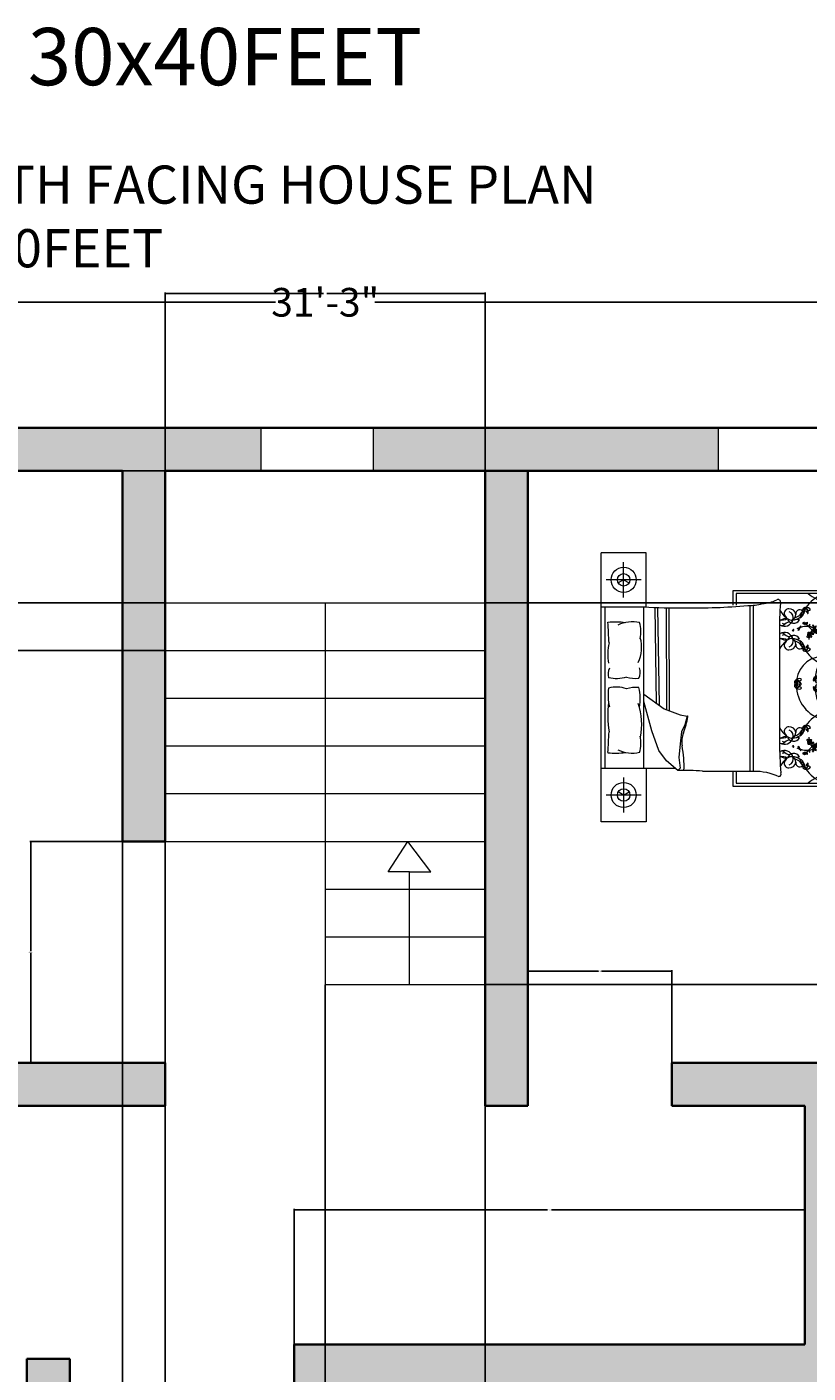
# Model space of a CAD drawing. Units: inches. Extents: x 8 to 486, y -516 to 97.
# Tile 4 of 5: x 162 to 326, y -185 to 97. Entities that reach past the tile are written whole.
import ezdxf

# ---------------------------------------------------------------- set-up
doc = ezdxf.new("R2010")
doc.units = ezdxf.units.IN
doc.header["$MEASUREMENT"] = 0
for name, color, linetype, lineweight in [('A-ANNO-DIMS', 2, 'Continuous', 18), ('A-ANNO-TEXT', 7, 'Continuous', 25), ('A-FLOR-STRS', 7, 'Continuous', 18), ('A-FURN', 8, 'Continuous', 18), ('A-GLAZ', 4, 'Continuous', 18), ('A-WALL', 7, 'Continuous', 35), ('A-WALL-PATT', 150, 'Continuous', 13)]:
    doc.layers.add(name, color=color, linetype=linetype, lineweight=lineweight)
doc.styles.get("Standard").update_dxf_attribs({"font": 'arial.ttf'})
doc.dimstyles.get("Standard").update_dxf_attribs({"dimtxt": 0.18, "dimasz": 0.18, "dimexe": 0.18, "dimexo": 0.0625, "dimgap": 0.09, "dimtad": 0, "dimtih": 1, "dimtoh": 1, "dimdec": 0, "dimzin": 0, "dimdsep": 46, "dimlunit": 3, "dimtxsty": 'Standard', "dimcen": 0.09, "dimadec": 0, "dimazin": 0, "dimtfac": 1, "dimtdec": 0, "dimtofl": 0, "dimtmove": 0, "dimatfit": 3, "dimfxl": 1, "dimtolj": 1, "dimtzin": 0, "dimarcsym": 0})

# ---------------------------------------------------------------- blocks, each defined once
blk = doc.blocks.new('*D1')
at = {"layer": 'A-ANNO-DIMS', "color": 0, "lineweight": -2, "transparency": 16777216}
for p, q in [((37.13, 12.8), (37.13, 39.25)), ((37.31, 39.07), (214.23, 39.07)), ((411.95, 39.07), (235.02, 39.07)), ((412.13, 12.8), (412.13, 39.25))]:
    blk.add_line(p, q, dxfattribs=at)
at = {"layer": 'A-ANNO-DIMS', "color": 0, "transparency": 16777216}
for points in [[(37.31, 39.1), (37.31, 39.04), (37.13, 39.07)], [(411.95, 39.1), (411.95, 39.04), (412.13, 39.07)]]:
    blk.add_solid(points, dxfattribs=at)
at = {"layer": 'Defpoints', "color": 0, "transparency": 16777216}
for p in [(412.13, 39.07), (37.13, 12.74), (412.13, 12.74)]:
    blk.add_point(p, dxfattribs=at)
at = {"layer": 'A-ANNO-DIMS', "color": 0, "transparency": 16777216, "insert": (224.63, 39.07), "char_height": 6, "attachment_point": 5}
blk.add_mtext('\\A1;31\'-3"', dxfattribs=at)
blk = doc.blocks.new('BED-DOUBLE')
for p, q in [((0, 0), (0, 56.34)), ((4.7, 47.03), (4.7, 54.39)), ((8.38, 50.71), (1.01, 50.71)), ((27.62, 45.39), (27.62, 48.51)), ((27.62, 48.51), (47.92, 48.51)), ((47.92, 48.51), (47.92, 7.44)), ((28.27, 47.86), (28.27, 45.37)), ((47.26, 47.86), (28.27, 47.86)), ((31.13, 45.33), (31.13, 10.62)), ((31.84, 45.38), (31.84, 10.62)), ((47.26, 8.09), (47.26, 47.86)), ((0.72, 45.07), (0.72, 11.27)), ((8.9, 11.27), (8.9, 45.07)), ((11.24, 44.92), (11.53, 24.86)), ((11.82, 44.9), (12.11, 24.44)), ((13.6, 44.87), (13.68, 23.48)), ((14.18, 44.87), (14.26, 23.26)), ((41.55, 42.31), (40.91, 42.43)), ((37.37, 39.61), (37.37, 16.73)), ((41.55, 38.37), (40.91, 38.24)), ((8.9, 26.75), (13.2, 23.66)), ((10.58, 19.09), (8.9, 25.24)), ((13.2, 23.66), (16.51, 22.4)), ((16.51, 22.4), (17.99, 22.17)), ((17.54, 20.35), (16.85, 18.87)), ((17.99, 22.17), (17.54, 20.35)), ((12.06, 14.99), (10.58, 19.09)), ((16.85, 18.87), (16.51, 16.36)), ((41.55, 17.58), (40.91, 17.7)), ((13.66, 12.82), (12.06, 14.99)), ((16.51, 16.36), (16.28, 13.5)), ((16.05, 10.76), (13.66, 12.82)), ((16.28, 13.5), (16.51, 11.22)), ((41.55, 13.64), (40.91, 13.52)), ((0, 11.27), (15.46, 11.27)), ((4.7, 9.31), (4.7, 1.95)), ((16.51, 11.22), (16.05, 10.76)), ((27.62, 7.44), (27.62, 10.62)), ((28.27, 10.62), (28.27, 8.09)), ((47.92, 7.44), (27.62, 7.44)), ((28.27, 8.09), (47.26, 8.09)), ((8.38, 5.63), (1.01, 5.63))]:
    blk.add_line(p, q)
for points in [[(0, 45.07), (9.39, 45.07), (9.39, 56.34), (0, 56.34)], [(4.7, 50.71), (3.56, 50.05)], [(4.7, 50.71), (5.83, 50.05)], [(9.39, 11.27), (9.39, 0), (0, 0)], [(4.7, 5.63), (3.56, 6.29)], [(4.7, 5.63), (5.83, 6.29)]]:
    blk.add_lwpolyline(points)
for points in [[(30.69, 45.31, 0.056112), (33.79, 45.72, 0.095341), (36.78, 46.51)], [(1.4, 41.84, -0.074897), (5.08, 41.77, 0.472817)], [(5.29, 30.31, -0.14099), (1.54, 30.2, -0.235245)], [(5.29, 27.91, 0.14099), (1.54, 28.02, 0.235245)], [(1.4, 14.5, 0.074897), (5.08, 14.57, -0.472817)], [(21.21, 10.65, 0.001242), (31.9, 10.62, -0.127202), (37.23, 9.49)]]:
    blk.add_lwpolyline(points, format="xyb")
for centre, radius in [((4.7, 50.71), 2.63), ((4.7, 50.71), 1.31), ((45.1, 39.99), 0.143), ((43.59, 39.05), 0.143), ((43.59, 16.9), 0.143), ((45.1, 15.96), 0.143), ((4.7, 5.63), 2.63), ((4.7, 5.63), 1.31)]:
    blk.add_circle(centre, radius)
for centre, radius, start, end in [((19.47, 176.89), 132.06, 269.1145, 274.8735), ((37.06, 46.09), 0.514, 336.5219, 123.8264), ((92.17, 41.33), 54.82, 175.2402, 181.8035), ((48.98, 40.75), 7.36, 111.4092, 145.6135), ((48.25, 53.34), 7.36, 228.1144, 262.255), ((49.24, 49.64), 3.59, 209.8884, 236.5383), ((48.41, 47.64), 2.99, 221.0454, 247.4453), ((46.8, 55.83), 10.18, 266.3481, 272.5919), ((49.91, 50.93), 4.47, 223.5186, 233.6964), ((15.79, 146.07), 101.24, 266.1, 270.9282), ((37.79, 44.6), 2.33, 259.249, 301.1782), ((41.34, 46.16), 4.26, 203.6453, 236.3329), ((38.8, 40.44), 2.17, 85.2696, 124.215), ((39.29, 43.68), 0.951, 88.9462, 185.5144), ((39.99, 43.97), 1.69, 193.079, 274.7067), ((40.34, 43), 1.4, 196.8663, 330.0915), ((39.43, 43.29), 1.35, 7.1143, 95.0551), ((38.92, 42.76), 1.31, 338.5779, 68.4181), ((39.13, 43.52), 1.64, 305.9599, 357.6409), ((39.95, 45.3), 3.02, 273.4924, 303.7117), ((39.73, 45.27), 2.66, 288.2955, 328.7386), ((41.6, 43.6), 0.846, 19.1312, 189.736), ((41.34, 43.8), 1.06, 285.6955, 4.031), ((42.75, 42.66), 1.12, 128.4175, 173.8338), ((42.51, 43.77), 0.518, 126.7319, 206.0245), ((42.76, 44.31), 0.61, 76.272, 177.0484), ((41.84, 45.56), 1.26, 284.7031, 328.6173), ((43.59, 43.96), 1.16, 125.7657, 194.5347), ((37.88, 46.02), 5.15, 332.8176, 347.4827), ((43.08, 44.11), 0.816, 20.9613, 102.2885), ((43.52, 44.92), 0.614, 181.7131, 301.5367), ((41.51, 43.68), 1.86, 2.0648, 41.1598), ((42.63, 44.37), 0.602, 316.2238, 62.3173), ((42.98, 44.02), 0.048, 20.2667, 316.2271), ((43.23, 43.75), 0.0444, 52.0591, 168.5166), ((43.28, 43.74), 0.0914, 168.5166, 2.0648), ((-534.78, 10.78), 537.08, 2.8502, 3.3148), ((6.56, 34.66), 7.26, 78.2417, 114.8684), ((0.75, 39.83), 7.55, 348.9631, 14.8961), ((37.99, 41.7), 0.679, 196.6343, 225.5483), ((37.99, 41.7), 0.679, 127.675, 162.5814), ((38.39, 42.79), 1.8, 240.8249, 340.7178), ((37.86, 41.99), 0.843, 246.1646, 318.4347), ((38.39, 37.89), 1.8, 19.2822, 119.1751), ((37.86, 38.68), 0.843, 41.5653, 113.8354), ((38.72, 43.06), 1.62, 240.0851, 262.564), ((39.35, 40.67), 1.16, 74.8529, 138.4347), ((39.75, 42.12), 0.35, 254.8529, 12.6959), ((38.8, 40.44), 2.17, 53.6555, 57.2989), ((40.21, 40.19), 0.177, 169.5864, 349.5616), ((40.28, 40.18), 0.109, 349.5616, 167.2949), ((43.11, 36.27), 4.67, 110.1059, 116.9968), ((41.55, 40.12), 0.296, 129.5056, 182.6421), ((40.7, 40.8), 0.89, 308.4388, 328.836), ((40.54, 41.53), 1.59, 296.5064, 305.3102), ((40.53, 40.71), 0.905, 336.3901, 344.4871), ((41.52, 40.48), 0.115, 83.9457, 185.6216), ((41.06, 40.58), 0.472, 328.836, 0.8141), ((41.3, 40.45), 0.27, 306.5232, 32.4668), ((41.62, 40.66), 0.115, 112.5583, 214.2343), ((41.55, 40.86), 0.27, 265.7131, 351.6568), ((41.31, 41.01), 0.472, 297.3659, 329.344), ((40.95, 41.42), 0.905, 313.6929, 321.7899), ((41.96, 40.8), 0.296, 115.5379, 168.6744), ((40.95, 41.22), 0.89, 329.344, 349.7412), ((43.11, 36.27), 4.67, 86.1723, 106.4158), ((40.24, 41.02), 1.59, 352.8698, 1.6736), ((42.35, 41.59), 0.111, 125.0752, 284.7644), ((42.52, 41.63), 0.239, 127.3642, 168.4363), ((42.33, 41.83), 0.345, 277.4968, 341.2737), ((42.6, 41.67), 0.137, 88.1325, 178.8919), ((42.88, 41.52), 0.297, 136.3462, 189.6513), ((42.71, 41.49), 0.124, 189.6513, 312.3208), ((42.74, 41.83), 0.143, 183.2768, 356.7232), ((43.19, 41.58), 0.47, 164.2829, 186.9148), ((42.63, 41.57), 0.235, 312.3208, 40.2111), ((43.13, 41.84), 0.333, 201.6382, 274.947), ((42.69, 41.38), 0.436, 42.3896, 66.5724), ((47.08, 44.83), 5.35, 217.9541, 226.8459), ((43, 41.64), 0.237, 10.9597, 52.2379), ((43.15, 41.62), 0.11, 274.947, 37.5263), ((43.38, 40.15), 0.654, 253.6301, 325.4631), ((43.56, 39.24), 0.463, 82.0748, 142.6895), ((43.51, 39.88), 0.475, 228.342, 274.9894), ((43.52, 40.99), 0.115, 112.5583, 214.2343), ((43.45, 41.2), 0.27, 265.7131, 351.6568), ((43.21, 41.35), 0.472, 297.3659, 329.344), ((43.23, 38.6), 2.34, 60.7959, 85.244), ((38.25, 35.23), 7.7, 37.8256, 47.7588), ((42.85, 41.75), 0.905, 313.6929, 321.7899), ((43.52, 39.8), 0.398, 273.8774, 357.1501), ((43.85, 41.13), 0.296, 115.5379, 168.6744), ((42.85, 41.56), 0.89, 329.344, 349.7412), ((43.68, 40.08), 0.385, 262.0748, 308.2393), ((42.14, 41.35), 1.59, 352.8698, 1.6736), ((46.34, 38.35), 2.81, 156.1523, 156.9499), ((43.86, 39.35), 0.142, 44.3732, 121.9501), ((44.3, 39.69), 0.398, 181.4625, 249.4747), ((46.34, 38.35), 2.81, 130.182, 149.456), ((44.23, 40), 0.385, 215.1128, 261.2773), ((44.54, 39.98), 0.654, 197.889, 269.722), ((44.1, 39.16), 0.463, 20.6625, 81.2773), ((44.37, 41.03), 0.16, 33.0979, 123.1364), ((40.84, 38.77), 4.19, 31.1156, 34.8118), ((44.14, 40.76), 0.434, 2.3172, 70.5201), ((44.79, 39.95), 0.463, 139.3812, 199.9959), ((43.93, 40.29), 0.654, 310.9365, 22.7695), ((44.23, 40.25), 0.475, 285.6484, 332.2957), ((44.5, 40.65), 0.125, 135.7354, 318.1297), ((44.29, 40.86), 0.166, 315.7354, 31.1156), ((44.15, 40.5), 0.385, 319.3812, 5.5456), ((44.59, 40.65), 0.125, 68.2452, 250.6395), ((44.3, 40.81), 0.374, 352.6008, 57.1845), ((45.64, 38.3), 2.5, 111.7087, 116.2181), ((43.23, 38.6), 2.34, 47.5083, 55.9967), ((44.66, 40.89), 0.374, 252.8042, 349.6943), ((44.3, 40.22), 0.398, 331.1838, 51.6792), ((44.71, 39.75), 0.111, 125.0752, 284.7644), ((44.7, 40.92), 0.166, 248.2452, 323.6254), ((44.88, 39.79), 0.239, 93.635, 168.4363), ((44.55, 41.02), 0.434, 291.7087, 3.0299), ((44.85, 40.17), 0.141, 138.2946, 276.2474), ((44.69, 39.98), 0.345, 277.4968, 341.2737), ((44.9, 40.15), 0.196, 358.5719, 143.8954), ((41.46, 43.31), 4.19, 323.6254, 327.3216), ((44.97, 39.82), 0.137, 88.1325, 178.8919), ((45.02, 40.3), 0.197, 208.8493, 269.9355), ((44.85, 40.26), 0.226, 274.2123, 318.1587), ((45.24, 39.68), 0.297, 136.3462, 189.6513), ((45.07, 39.65), 0.124, 189.6513, 312.3208), ((44.89, 40.92), 0.16, 325.6077, 55.6462), ((45.55, 39.73), 0.47, 164.2829, 186.9148), ((45.54, 40.03), 0.452, 121.9501, 165.2442), ((45, 39.73), 0.235, 312.3208, 40.2111), ((45.5, 39.99), 0.333, 201.6382, 274.947), ((45.23, 40.2), 0.095, 262.868, 7.094), ((45.05, 39.54), 0.436, 42.3896, 66.5724), ((45.21, 40.28), 0.283, 278.5614, 22.5914), ((45.37, 39.79), 0.237, 10.9597, 118.7804), ((45.37, 40.29), 0.142, 44.3732, 121.9501), ((45.52, 39.77), 0.11, 274.947, 37.5263), ((11.26, 35.15), 9.9, 166.3427, 191.1841), ((1.3, 36.57), 7.17, 333.8761, 16.1746), ((37.99, 38.97), 0.679, 134.4517, 156.7144), ((37.99, 38.97), 0.679, 203.2856, 232.325), ((37.79, 36.08), 2.33, 58.8218, 100.2867), ((41.34, 34.52), 4.26, 123.6671, 158.5059), ((38.8, 40.23), 2.17, 235.785, 274.7304), ((38.72, 37.62), 1.62, 97.436, 119.9149), ((39.99, 36.71), 1.69, 85.2933, 166.921), ((39.29, 37), 0.951, 174.4856, 271.0538), ((39.35, 40.01), 1.16, 221.5653, 285.1471), ((40.34, 37.67), 1.4, 29.9085, 163.1337), ((39.43, 37.39), 1.35, 264.9449, 352.8857), ((38.92, 37.92), 1.31, 291.5819, 21.4221), ((39.75, 38.56), 0.35, 347.3041, 105.1471), ((38.8, 40.23), 2.17, 302.7011, 306.3445), ((39.13, 37.16), 1.64, 2.3591, 54.0401), ((39.95, 35.38), 3.02, 56.2883, 86.5076), ((39.73, 35.4), 2.66, 31.2614, 71.7045), ((41.6, 37.08), 0.846, 170.264, 340.8688), ((42.75, 38.01), 1.12, 186.1662, 231.5825), ((41.34, 36.88), 1.06, 355.969, 74.3045), ((42.51, 36.91), 0.518, 153.9755, 233.2681), ((43.59, 36.72), 1.16, 165.4653, 234.2343), ((37.88, 34.66), 5.15, 12.5173, 27.1824), ((41.51, 37), 1.86, 318.8402, 357.9352), ((42.63, 36.3), 0.602, 297.6827, 43.7762), ((43.01, 36.67), 0.0796, 43.7762, 339.7183), ((43.2, 38.81), 0.111, 125.0752, 284.7644), ((43.37, 38.85), 0.239, 93.635, 168.4363), ((43.28, 36.93), 0.0914, 357.9352, 191.4834), ((43.23, 36.92), 0.0444, 191.4834, 307.9409), ((43.34, 39.23), 0.141, 138.2946, 276.2474), ((43.39, 39.21), 0.196, 358.5719, 143.8954), ((43.18, 39.05), 0.345, 277.4968, 341.2737), ((43.46, 38.88), 0.137, 88.1325, 178.8919), ((43.51, 39.36), 0.197, 208.8493, 269.9355), ((43.34, 39.32), 0.226, 274.2123, 318.1587), ((43.73, 38.74), 0.297, 136.3462, 189.6513), ((43.56, 38.71), 0.124, 189.6513, 312.3208), ((46.34, 38.35), 2.81, 175.2415, 182.8929), ((44.04, 38.79), 0.47, 164.2829, 186.9148), ((44.03, 39.09), 0.452, 121.9501, 165.2442), ((43.49, 38.79), 0.235, 312.3208, 40.2111), ((43.98, 39.06), 0.333, 201.6382, 274.947), ((43.71, 39.26), 0.095, 262.868, 7.094), ((43.54, 38.6), 0.436, 42.3896, 66.5724), ((43.7, 39.34), 0.283, 278.5614, 22.5914), ((43.86, 38.86), 0.237, 10.9597, 118.7804), ((44, 38.83), 0.11, 274.947, 37.5263), ((44.34, 39.76), 0.475, 248.3627, 295.0101), ((46.55, 28.98), 5.69, 82.8636, 171.8197), ((42.76, 36.36), 0.61, 182.9516, 283.728), ((41.84, 35.12), 1.26, 31.3827, 75.2969), ((43.52, 35.75), 0.614, 58.4633, 178.2869), ((43.08, 36.57), 0.816, 257.7115, 339.0387), ((48.98, 39.93), 7.36, 214.3865, 248.5908), ((46.95, 32.74), 1.32, 76.3898, 169.0739), ((48.41, 33.04), 2.99, 112.5547, 138.9546), ((46.8, 24.84), 10.18, 87.4081, 93.6519), ((4.21, 30.97), 2.79, 153.3437, 196.1026), ((5.19, 31.35), 2.99, 335.0183, 18.5407), ((52.19, 29.78), 7.36, 152.5854, 175.5377), ((46.77, 31.74), 1.67, 72.8609, 131.9049), ((46.03, 29.72), 3.29, 68.117, 96.6195), ((51.13, 31.84), 4.05, 162.9798, 196.4569), ((7.17, 36.95), 6.9, 254.1707, 275.9871), ((41.09, 29.2), 0.61, 106.1963, 206.9726), ((41.09, 28.62), 0.61, 153.0274, 253.8037), ((39.66, 29.82), 1.26, 314.6273, 358.5415), ((39.66, 28), 1.26, 1.4585, 45.3727), ((41.98, 29.31), 1.16, 155.6899, 224.4589), ((41.98, 28.51), 1.16, 135.5411, 204.3101), ((41.47, 29.19), 0.816, 50.8855, 132.2127), ((41.44, 30.11), 0.614, 211.6373, 331.4609), ((40.94, 29.19), 0.602, 346.148, 92.2415), ((40.32, 28.03), 1.86, 31.989, 71.0841), ((36.01, 28.25), 5.15, 2.7418, 17.407), ((36.01, 29.58), 5.15, 342.593, 357.2582), ((40.32, 29.8), 1.86, 288.9159, 328.011), ((40.94, 28.64), 0.602, 267.7585, 13.852), ((41.44, 27.71), 0.614, 28.5391, 148.3627), ((41.42, 29.06), 0.048, 50.1909, 346.0209), ((41.45, 28.76), 0.0796, 13.852, 309.9245), ((41.82, 28.97), 0.0914, 198.4408, 31.989), ((41.77, 28.95), 0.0444, 81.9833, 198.4408), ((41.82, 28.86), 0.0914, 328.011, 161.5592), ((41.77, 28.87), 0.0444, 161.5592, 278.0167), ((45.03, 29.77), 0.61, 106.1963, 206.9726), ((45.03, 28.06), 0.61, 153.0274, 253.8037), ((43.6, 30.38), 1.26, 314.6273, 358.5415), ((43.6, 27.44), 1.26, 1.4585, 45.3727), ((45.92, 29.87), 1.16, 155.6899, 224.4589), ((45.92, 27.95), 1.16, 135.5411, 204.3101), ((45.41, 29.75), 0.816, 50.8855, 132.2127), ((45.38, 30.68), 0.614, 211.6373, 331.4609), ((44.26, 28.59), 1.86, 31.989, 71.0841), ((39.95, 28.81), 5.15, 2.7418, 17.407), ((44.88, 29.75), 0.602, 346.148, 92.2415), ((39.95, 29.01), 5.15, 342.593, 357.2582), ((44.26, 29.23), 1.86, 288.9159, 328.011), ((44.88, 28.07), 0.602, 267.7585, 13.852), ((45.36, 29.62), 0.048, 50.1909, 346.0209), ((45.39, 28.2), 0.0796, 13.852, 309.9245), ((45.76, 29.53), 0.0914, 198.4408, 31.989), ((45.71, 29.52), 0.0444, 81.9833, 198.4408), ((45.76, 28.3), 0.0914, 328.011, 161.5592), ((45.71, 28.31), 0.0444, 161.5592, 278.0167), ((53.22, 30.24), 5.98, 174.3643, 175.6213), ((57.31, 27.08), 10.69, 160.0972, 160.2783), ((11.47, 26.54), 10.04, 171.5249, 193.96), ((7.17, 21.26), 6.9, 84.0129, 105.8293), ((-1.76, 25.79), 9.94, 349.8617, 13.6238), ((41.47, 28.64), 0.816, 227.7873, 309.1145), ((48.25, 28.61), 7.36, 184.4623, 262.255), ((45.38, 27.15), 0.614, 28.5391, 148.3627), ((45.41, 28.08), 0.816, 227.7873, 309.1145), ((52.19, 28.04), 7.36, 184.4623, 207.4146), ((51.13, 25.99), 4.05, 163.5431, 197.0202), ((53.22, 27.59), 5.98, 184.3787, 185.6357), ((57.31, 30.74), 10.69, 199.7217, 199.9028), ((21.79, 22.22), 20.43, 172.2196, 189.497), ((-4.62, 20.49), 13.1, 348.0397, 19.2615), ((48.98, 16.02), 7.36, 111.4092, 145.6135), ((49.24, 24.92), 3.59, 181.272, 236.5383), ((51.16, 28.56), 6.65, 214.0123, 234.053), ((49.91, 26.21), 4.47, 197.8504, 233.6964), ((-3.3, 26.09), 21.85, 340.1194, 349.3383), ((18.04, 22.05), 0.136, 358.8623, 109.7536), ((41.34, 21.43), 4.26, 201.4941, 236.3329), ((39.29, 18.95), 0.951, 88.9462, 185.5144), ((39.43, 18.56), 1.35, 7.1143, 95.0551), ((42.76, 19.58), 0.61, 76.272, 177.0484), ((41.84, 20.83), 1.26, 284.7031, 328.6173), ((43.59, 19.23), 1.16, 125.7657, 194.5347), ((37.88, 21.29), 5.15, 332.8176, 347.4827), ((43.08, 19.38), 0.816, 20.9613, 102.2885), ((42.63, 19.64), 0.602, 316.2238, 62.3173), ((41.51, 18.95), 1.86, 2.0648, 41.1598), ((43.52, 20.19), 0.614, 181.7131, 301.5367), ((46.8, 31.1), 10.18, 266.3481, 272.5919), ((48.41, 22.91), 2.99, 221.0454, 247.4453), ((-534.78, 45.56), 537.08, 356.6852, 357.1498), ((0.75, 16.51), 7.55, 345.1039, 11.0369), ((21.45, 16.81), 4.59, 156.2616, 191.3392), ((37.79, 19.87), 2.33, 259.7133, 301.1782), ((37.99, 16.98), 0.679, 127.675, 156.7144), ((38.39, 18.06), 1.8, 240.8249, 340.7178), ((38.8, 15.72), 2.17, 85.2696, 124.215), ((38.72, 18.33), 1.62, 240.0851, 262.564), ((39.99, 19.24), 1.69, 193.079, 274.7067), ((39.35, 15.94), 1.16, 74.8529, 138.4347), ((40.34, 18.28), 1.4, 196.8663, 330.0915), ((38.92, 18.03), 1.31, 338.5779, 68.4181), ((39.75, 17.39), 0.35, 254.8529, 12.6959), ((38.8, 15.72), 2.17, 53.6555, 57.2989), ((39.13, 18.79), 1.64, 305.9599, 357.6409), ((39.95, 20.57), 3.02, 273.4924, 303.7117), ((39.73, 20.54), 2.66, 288.2955, 328.7386), ((41.6, 18.87), 0.846, 19.1312, 189.736), ((41.34, 19.07), 1.06, 285.6955, 4.031), ((42.75, 17.93), 1.12, 128.4175, 173.8338), ((42.51, 19.04), 0.518, 126.7319, 206.0245), ((42.98, 19.29), 0.048, 20.2667, 316.2271), ((43.2, 17.14), 0.111, 75.2356, 234.9248), ((43.37, 17.09), 0.239, 191.5637, 266.365), ((43.23, 19.02), 0.0444, 52.0591, 168.5166), ((43.28, 19.02), 0.0914, 168.5166, 2.0648), ((43.18, 16.9), 0.345, 18.7263, 82.5032), ((43.46, 17.06), 0.137, 181.1081, 271.8675), ((43.73, 17.21), 0.297, 170.3487, 223.6538), ((43.56, 17.24), 0.124, 47.6792, 170.3487), ((46.34, 17.59), 2.81, 177.1071, 184.7585), ((44.04, 17.15), 0.47, 173.0852, 195.7171), ((43.49, 17.16), 0.235, 319.7889, 47.6792), ((43.98, 16.89), 0.333, 85.053, 158.3618), ((43.54, 17.35), 0.436, 293.4276, 317.6104), ((43.86, 17.09), 0.237, 241.2196, 349.0403), ((44, 17.11), 0.11, 322.4737, 85.053), ((6.56, 21.68), 7.26, 245.1316, 281.7583), ((-3.9, 11.73), 21.26, 357.4519, 11.3392), ((96.02, 16.06), 58.65, 179.3433, 185.6887), ((37.99, 16.98), 0.679, 203.229, 225.5483), ((37.99, 14.24), 0.679, 134.4517, 153.558), ((37.86, 17.26), 0.843, 246.1646, 318.4347), ((38.39, 13.16), 1.8, 19.2822, 119.1751), ((37.86, 13.96), 0.843, 41.5653, 113.8354), ((38.72, 12.89), 1.62, 97.436, 119.9149), ((39.35, 15.28), 1.16, 221.5653, 285.1471), ((40.34, 12.94), 1.4, 29.9085, 163.1337), ((39.75, 13.83), 0.35, 347.3041, 105.1471), ((40.21, 15.76), 0.177, 10.4384, 190.4136), ((40.28, 15.77), 0.109, 192.7051, 10.4384), ((43.11, 19.68), 4.67, 243.0032, 249.8941), ((40.7, 15.15), 0.89, 31.164, 51.5612), ((41.55, 15.83), 0.296, 177.3579, 230.4944), ((40.54, 14.42), 1.59, 54.6898, 63.4936), ((40.53, 15.24), 0.905, 15.5129, 23.6099), ((41.52, 15.47), 0.115, 174.3784, 276.0543), ((41.3, 15.5), 0.27, 327.5332, 53.4768), ((41.06, 15.36), 0.472, 359.1859, 31.164), ((41.62, 15.29), 0.115, 145.7657, 247.4417), ((41.55, 15.09), 0.27, 8.3432, 94.2869), ((41.31, 14.94), 0.472, 30.656, 62.6341), ((40.95, 14.53), 0.905, 38.2101, 46.3071), ((41.96, 15.15), 0.296, 191.3256, 244.4621), ((40.95, 14.72), 0.89, 10.2588, 30.656), ((43.11, 19.68), 4.67, 253.5842, 273.8277), ((40.24, 14.93), 1.59, 358.3264, 7.1302), ((42.35, 14.36), 0.111, 75.2356, 234.9248), ((42.52, 14.31), 0.239, 191.5637, 232.6358), ((42.33, 14.12), 0.345, 18.7263, 82.5032), ((42.6, 14.28), 0.137, 181.1081, 271.8675), ((42.88, 14.43), 0.297, 170.3487, 223.6538), ((42.71, 14.46), 0.124, 47.6792, 170.3487), ((42.74, 14.11), 0.143, 3.2768, 176.7232), ((43.19, 14.37), 0.47, 173.0852, 195.7171), ((42.63, 14.37), 0.235, 319.7889, 47.6792), ((43.13, 14.11), 0.333, 85.053, 158.3618), ((42.69, 14.57), 0.436, 293.4276, 317.6104), ((47.08, 11.12), 5.35, 133.1541, 142.0459), ((43, 14.31), 0.237, 307.7621, 349.0403), ((43.15, 14.33), 0.11, 322.4737, 85.053), ((43.51, 16.07), 0.475, 85.0106, 131.658), ((43.38, 15.8), 0.654, 34.5369, 106.3699), ((43.56, 16.71), 0.463, 217.3105, 277.9252), ((43.34, 16.72), 0.141, 83.7526, 221.7054), ((43.39, 16.74), 0.196, 216.1046, 1.4281), ((43.51, 16.58), 0.197, 90.0645, 151.1507), ((43.34, 16.63), 0.226, 41.8413, 85.7877), ((43.52, 14.96), 0.115, 145.7657, 247.4417), ((38.25, 20.72), 7.7, 312.2412, 322.1744), ((43.23, 17.35), 2.34, 274.756, 299.2041), ((43.45, 14.75), 0.27, 8.3432, 94.2869), ((43.21, 14.6), 0.472, 30.656, 62.6341), ((42.85, 14.2), 0.905, 38.2101, 46.3071), ((43.52, 16.15), 0.398, 2.8499, 86.1226), ((43.85, 14.81), 0.296, 191.3256, 244.4621), ((44.03, 16.86), 0.452, 194.7558, 238.0499), ((42.85, 14.39), 0.89, 10.2588, 30.656), ((43.68, 15.87), 0.385, 51.7607, 97.9252), ((43.71, 16.68), 0.095, 352.906, 97.132), ((42.14, 14.59), 1.59, 358.3264, 7.1302), ((43.7, 16.6), 0.283, 337.4086, 81.4386), ((46.34, 17.59), 2.81, 203.0501, 203.8477), ((43.86, 16.59), 0.142, 238.0499, 315.6268), ((44.3, 16.26), 0.398, 110.5253, 178.5375), ((44.54, 15.97), 0.654, 90.278, 162.111), ((44.23, 15.95), 0.385, 98.7227, 144.8872), ((46.34, 17.59), 2.81, 210.544, 229.818), ((44.34, 16.19), 0.475, 64.9899, 111.6373), ((44.1, 16.78), 0.463, 278.7227, 339.3375), ((44.14, 15.19), 0.434, 289.4799, 357.6828), ((40.84, 17.17), 4.19, 325.1882, 328.8844), ((44.37, 14.91), 0.16, 236.8636, 326.9021), ((44.79, 15.99), 0.463, 160.0041, 220.6188), ((43.93, 15.66), 0.654, 337.2305, 49.0635), ((44.23, 15.7), 0.475, 27.7043, 74.3516), ((44.5, 15.3), 0.125, 41.8703, 224.2646), ((44.29, 15.09), 0.166, 328.8844, 44.2646), ((44.15, 15.44), 0.385, 354.4544, 40.6188), ((44.59, 15.29), 0.125, 109.3605, 291.7548), ((44.3, 15.14), 0.374, 302.8155, 7.3992), ((45.64, 17.65), 2.5, 243.7819, 248.2913), ((43.23, 17.35), 2.34, 304.0033, 312.4917), ((44.3, 15.72), 0.398, 308.3208, 28.8162), ((44.66, 15.06), 0.374, 10.3057, 107.1958), ((44.71, 16.2), 0.111, 75.2356, 234.9248), ((44.7, 15.02), 0.166, 36.3746, 111.7548), ((44.88, 16.16), 0.239, 191.5637, 266.365), ((44.85, 15.78), 0.141, 83.7526, 221.7054), ((44.55, 14.92), 0.434, 356.9701, 68.2913), ((44.69, 15.96), 0.345, 18.7263, 82.5032), ((44.9, 15.8), 0.196, 216.1046, 1.4281), ((44.97, 16.12), 0.137, 181.1081, 271.8675), ((41.46, 12.64), 4.19, 32.6784, 36.3746), ((45.02, 15.65), 0.197, 90.0645, 151.1507), ((44.85, 15.69), 0.226, 41.8413, 85.7877), ((45.07, 16.3), 0.124, 47.6792, 170.3487), ((45.24, 16.27), 0.297, 170.3487, 223.6538), ((44.89, 15.03), 0.16, 304.3538, 34.3923), ((45.55, 16.21), 0.47, 173.0852, 195.7171), ((45.54, 15.92), 0.452, 194.7558, 238.0499), ((45, 16.22), 0.235, 319.7889, 47.6792), ((45.5, 15.95), 0.333, 85.053, 158.3618), ((45.23, 15.75), 0.095, 352.906, 97.132), ((45.05, 16.41), 0.436, 293.4276, 317.6104), ((45.37, 16.15), 0.237, 241.2196, 349.0403), ((45.21, 15.67), 0.283, 337.4086, 81.4386), ((45.37, 15.66), 0.142, 238.0499, 315.6268), ((45.52, 16.18), 0.11, 322.4737, 85.053), ((37.99, 14.24), 0.679, 210.0293, 232.325), ((37.79, 11.35), 2.33, 58.8218, 99.1554), ((41.34, 9.79), 4.26, 123.6671, 153.2997), ((38.8, 15.5), 2.17, 235.785, 274.7304), ((39.99, 11.98), 1.69, 85.2933, 166.921), ((39.29, 12.27), 0.951, 174.4856, 271.0538), ((39.43, 12.66), 1.35, 264.9449, 352.8857), ((38.92, 13.19), 1.31, 291.5819, 21.4221), ((38.8, 15.5), 2.17, 302.7011, 306.3445), ((39.13, 12.43), 1.64, 2.3591, 54.0401), ((39.95, 10.65), 3.02, 56.2883, 86.5076), ((39.73, 10.68), 2.66, 31.2614, 71.7045), ((41.6, 12.35), 0.846, 170.264, 340.8688), ((41.34, 12.15), 1.06, 355.969, 74.3045), ((42.75, 13.29), 1.12, 186.1662, 231.5825), ((42.51, 12.18), 0.518, 153.9755, 233.2681), ((41.84, 10.39), 1.26, 31.3827, 75.2969), ((42.76, 11.64), 0.61, 182.9516, 283.728), ((43.59, 11.99), 1.16, 165.4653, 234.2343), ((37.88, 9.93), 5.15, 12.5173, 27.1824), ((41.51, 12.27), 1.86, 318.8402, 357.9352), ((42.63, 11.58), 0.602, 297.6827, 43.7762), ((43.52, 11.03), 0.614, 58.4633, 178.2869), ((43.08, 11.84), 0.816, 257.7115, 339.0387), ((43.01, 11.94), 0.0796, 43.7762, 339.7183), ((43.28, 12.2), 0.0914, 357.9352, 191.4834), ((43.23, 12.2), 0.0444, 191.4834, 307.9409), ((17.45, -40.9), 51.68, 85.8294, 91.553), ((37.19, 10.01), 0.52, 273.98, 27.3412), ((48.98, 15.2), 7.36, 214.3865, 248.5908), ((48.25, 2.61), 7.36, 97.745, 131.8856), ((49.24, 6.3), 3.59, 123.4617, 150.1116), ((48.41, 8.31), 2.99, 112.5547, 138.9546), ((46.8, 0.12), 10.18, 87.4081, 93.6519), ((49.91, 5.01), 4.47, 126.3036, 136.4814)]:
    blk.add_arc(centre, radius, start, end)
blk = doc.blocks.new('*D27')
at = {"layer": 'A-ANNO-DIMS', "color": 0, "lineweight": -2, "transparency": 16777216}
for p, q in [((191.13, 3.8), (191.13, 41.12)), ((191.31, 40.94), (224.3, 40.94)), ((257.95, 40.94), (224.96, 40.94)), ((258.13, 3.8), (258.13, 41.12))]:
    blk.add_line(p, q, dxfattribs=at)
at = {"layer": 'A-ANNO-DIMS', "color": 0, "transparency": 16777216}
for points in [[(191.31, 40.97), (191.31, 40.91), (191.13, 40.94)], [(257.95, 40.97), (257.95, 40.91), (258.13, 40.94)]]:
    blk.add_solid(points, dxfattribs=at)
at = {"layer": 'Defpoints', "color": 0, "transparency": 16777216}
for p in [(258.13, 40.94), (191.13, 3.74), (258.13, 3.74)]:
    blk.add_point(p, dxfattribs=at)
at = {"layer": 'A-ANNO-DIMS', "color": 0, "transparency": 16777216, "insert": (224.63, 40.94), "char_height": 0.18, "attachment_point": 5}
blk.add_mtext('\\A1;5\'-7"', dxfattribs=at)
blk = doc.blocks.new('*D28')
at = {"layer": 'A-ANNO-DIMS', "color": 0, "lineweight": -2, "transparency": 16777216}
for p, q in [((191.06, -23.87), (8.75, -23.87)), ((8.93, -24.05), (8.93, -28.69)), ((8.93, -33.69), (8.93, -29.05)), ((191.06, -33.87), (8.75, -33.87))]:
    blk.add_line(p, q, dxfattribs=at)
at = {"layer": 'A-ANNO-DIMS', "color": 0, "transparency": 16777216}
for points in [[(8.9, -24.05), (8.96, -24.05), (8.93, -23.87)], [(8.9, -33.69), (8.96, -33.69), (8.93, -33.87)]]:
    blk.add_solid(points, dxfattribs=at)
at = {"layer": 'Defpoints', "color": 0, "transparency": 16777216}
for p in [(191.13, -23.87), (8.93, -33.87), (191.13, -33.87)]:
    blk.add_point(p, dxfattribs=at)
at = {"layer": 'A-ANNO-DIMS', "color": 0, "transparency": 16777216, "insert": (8.93, -28.87), "char_height": 0.18, "attachment_point": 5}
blk.add_mtext('\\A1;0\'-10"', dxfattribs=at)
blk = doc.blocks.new('*D29')
at = {"layer": 'A-ANNO-DIMS', "color": 0, "lineweight": -2, "transparency": 16777216}
for p, q in [((191.06, 3.74), (8.75, 3.74)), ((8.93, 3.56), (8.93, -9.89)), ((8.93, -23.69), (8.93, -10.25)), ((191.06, -23.87), (8.75, -23.87))]:
    blk.add_line(p, q, dxfattribs=at)
at = {"layer": 'A-ANNO-DIMS', "color": 0, "transparency": 16777216}
for points in [[(8.9, 3.56), (8.96, 3.56), (8.93, 3.74)], [(8.9, -23.69), (8.96, -23.69), (8.93, -23.87)]]:
    blk.add_solid(points, dxfattribs=at)
at = {"layer": 'Defpoints', "color": 0, "transparency": 16777216}
for p in [(191.13, 3.74), (8.93, -23.87), (191.13, -23.87)]:
    blk.add_point(p, dxfattribs=at)
at = {"layer": 'A-ANNO-DIMS', "color": 0, "transparency": 16777216, "insert": (8.93, -10.07), "char_height": 0.18, "attachment_point": 5}
blk.add_mtext('\\A1;2\'-3 1/2"', dxfattribs=at)
blk = doc.blocks.new('*D30')
at = {"layer": 'A-ANNO-DIMS', "color": 0, "lineweight": -2, "transparency": 16777216}
for p, q in [((224.63, -103.93), (224.63, -515.64)), ((258.13, -103.93), (258.13, -515.64)), ((224.81, -515.46), (240.84, -515.46)), ((257.95, -515.46), (241.92, -515.46))]:
    blk.add_line(p, q, dxfattribs=at)
at = {"layer": 'A-ANNO-DIMS', "color": 0, "transparency": 16777216}
for points in [[(224.81, -515.43), (224.81, -515.49), (224.63, -515.46)], [(257.95, -515.43), (257.95, -515.49), (258.13, -515.46)]]:
    blk.add_solid(points, dxfattribs=at)
at = {"layer": 'Defpoints', "color": 0, "transparency": 16777216}
for p in [(224.63, -103.87), (258.13, -103.87), (258.13, -515.46)]:
    blk.add_point(p, dxfattribs=at)
at = {"layer": 'A-ANNO-DIMS', "color": 0, "transparency": 16777216, "insert": (241.38, -515.46), "char_height": 0.18, "attachment_point": 5}
blk.add_mtext('\\A1;2\'-9 1/2"', dxfattribs=at)
blk = doc.blocks.new('*D31')
at = {"layer": 'A-ANNO-DIMS', "color": 0, "lineweight": -2, "transparency": 16777216}
for p, q in [((258.19, -23.87), (440.51, -23.87)), ((440.33, -24.05), (440.33, -63.69)), ((440.33, -103.69), (440.33, -64.05)), ((258.19, -103.87), (440.51, -103.87))]:
    blk.add_line(p, q, dxfattribs=at)
at = {"layer": 'A-ANNO-DIMS', "color": 0, "transparency": 16777216}
for points in [[(440.3, -24.05), (440.36, -24.05), (440.33, -23.87)], [(440.3, -103.69), (440.36, -103.69), (440.33, -103.87)]]:
    blk.add_solid(points, dxfattribs=at)
at = {"layer": 'Defpoints', "color": 0, "transparency": 16777216}
for p in [(258.13, -23.87), (258.13, -103.87), (440.33, -103.87)]:
    blk.add_point(p, dxfattribs=at)
at = {"layer": 'A-ANNO-DIMS', "color": 0, "transparency": 16777216, "insert": (440.33, -63.87), "char_height": 0.18, "attachment_point": 5}
blk.add_mtext('\\A1;6\'-8"', dxfattribs=at)
blk = doc.blocks.new('*D35')
at = {"layer": 'A-ANNO-DIMS', "color": 0, "lineweight": -2, "transparency": 16777216}
for p, q in [((182.13, -73.93), (182.13, -515.64)), ((191.13, -73.93), (191.13, -515.64)), ((182.31, -515.46), (186.3, -515.46)), ((190.95, -515.46), (186.96, -515.46))]:
    blk.add_line(p, q, dxfattribs=at)
at = {"layer": 'A-ANNO-DIMS', "color": 0, "transparency": 16777216}
for points in [[(182.31, -515.43), (182.31, -515.49), (182.13, -515.46)], [(190.95, -515.43), (190.95, -515.49), (191.13, -515.46)]]:
    blk.add_solid(points, dxfattribs=at)
at = {"layer": 'Defpoints', "color": 0, "transparency": 16777216}
for p in [(182.13, -73.87), (191.13, -73.87), (191.13, -515.46)]:
    blk.add_point(p, dxfattribs=at)
at = {"layer": 'A-ANNO-DIMS', "color": 0, "transparency": 16777216, "insert": (186.63, -515.46), "char_height": 0.18, "attachment_point": 5}
blk.add_mtext('\\A1;0\'-9"', dxfattribs=at)
blk = doc.blocks.new('*D38')
at = {"layer": 'A-ANNO-DIMS', "color": 0, "lineweight": -2, "transparency": 16777216}
for p, q in [((191.06, -73.87), (162.75, -73.87)), ((162.93, -74.05), (162.93, -96.89)), ((162.93, -120.08), (162.93, -97.25)), ((191.06, -120.26), (162.75, -120.26))]:
    blk.add_line(p, q, dxfattribs=at)
at = {"layer": 'A-ANNO-DIMS', "color": 0, "transparency": 16777216}
for points in [[(162.9, -74.05), (162.96, -74.05), (162.93, -73.87)], [(162.9, -120.08), (162.96, -120.08), (162.93, -120.26)]]:
    blk.add_solid(points, dxfattribs=at)
at = {"layer": 'Defpoints', "color": 0, "transparency": 16777216}
for p in [(162.93, -73.87), (191.13, -73.87), (191.13, -120.26)]:
    blk.add_point(p, dxfattribs=at)
at = {"layer": 'A-ANNO-DIMS', "color": 0, "transparency": 16777216, "insert": (162.93, -97.07), "char_height": 0.18, "attachment_point": 5}
blk.add_mtext('\\A1;3\'-10 1/2"', dxfattribs=at)
blk = doc.blocks.new('*D39')
at = {"layer": 'A-ANNO-DIMS', "color": 0, "lineweight": -2, "transparency": 16777216}
for p, q in [((267.13, -129.2), (267.13, -100.88)), ((267.31, -101.06), (281.88, -101.06)), ((297.11, -101.06), (282.54, -101.06)), ((297.29, -129.2), (297.29, -100.88))]:
    blk.add_line(p, q, dxfattribs=at)
at = {"layer": 'A-ANNO-DIMS', "color": 0, "transparency": 16777216}
for points in [[(267.31, -101.03), (267.31, -101.09), (267.13, -101.06)], [(297.11, -101.03), (297.11, -101.09), (297.29, -101.06)]]:
    blk.add_solid(points, dxfattribs=at)
at = {"layer": 'Defpoints', "color": 0, "transparency": 16777216}
for p in [(297.29, -101.06), (267.13, -129.26), (297.29, -129.26)]:
    blk.add_point(p, dxfattribs=at)
at = {"layer": 'A-ANNO-DIMS', "color": 0, "transparency": 16777216, "insert": (282.21, -101.06), "char_height": 0.18, "attachment_point": 5}
blk.add_mtext('\\A1;2\'-6"', dxfattribs=at)
blk = doc.blocks.new('*D41')
at = {"layer": 'A-ANNO-DIMS', "color": 0, "lineweight": -2, "transparency": 16777216}
for p, q in [((218.14, -179.2), (218.14, -150.88)), ((218.32, -151.06), (271.23, -151.06)), ((324.95, -151.06), (272.03, -151.06)), ((325.13, -179.2), (325.13, -150.88))]:
    blk.add_line(p, q, dxfattribs=at)
at = {"layer": 'A-ANNO-DIMS', "color": 0, "transparency": 16777216}
for points in [[(218.32, -151.03), (218.32, -151.09), (218.14, -151.06)], [(324.95, -151.03), (324.95, -151.09), (325.13, -151.06)]]:
    blk.add_solid(points, dxfattribs=at)
at = {"layer": 'Defpoints', "color": 0, "transparency": 16777216}
for p in [(325.13, -151.06), (218.14, -179.26), (325.13, -179.26)]:
    blk.add_point(p, dxfattribs=at)
at = {"layer": 'A-ANNO-DIMS', "color": 0, "transparency": 16777216, "insert": (271.63, -151.06), "char_height": 0.18, "attachment_point": 5}
blk.add_mtext('\\A1;8\'-11"', dxfattribs=at)

msp = doc.modelspace()

# ---------------------------------------------------------------- hatches: boundary and pattern name
at = {"layer": 'A-WALL-PATT'}
h = msp.add_hatch(color=256, dxfattribs=at)
h.dxf.hatch_style = 1
h.paths.add_polyline_path([(91.21, 12.74), (37.13, 12.74), (37.13, -29.65), (46.13, -29.65), (46.13, 3.74), (91.21, 3.74)])
h.paths.add_polyline_path([(211.13, 12.74), (137.85, 12.74), (137.85, 3.74), (182.13, 3.74), (182.13, -73.87), (191.13, -73.87), (191.13, 3.74), (211.13, 3.74)])
h.paths.add_polyline_path([(306.98, 12.74), (234.7, 12.74), (234.7, 3.74), (306.98, 3.74)])
h.paths.add_polyline_path([(267.13, 3.74), (258.13, 3.74), (258.13, -129.26), (267.13, -129.26)])
h.paths.add_polyline_path([(412.13, 12.74), (361.49, 12.74), (361.49, 3.74), (403.13, 3.74), (403.13, -35.28), (412.13, -35.28)])
h.paths.add_polyline_path([(379.01, -120.26), (297.29, -120.26), (297.29, -129.26), (325.13, -129.26), (325.13, -179.26), (218.14, -179.26), (218.14, -188.26), (325.13, -188.26), (325.13, -242.26), (297.29, -242.26), (297.29, -251.26), (379.01, -251.26), (379.01, -242.26), (334.13, -242.26), (334.13, -188.26), (403.13, -188.26), (403.13, -209.46), (412.13, -209.46), (412.13, -162.44), (403.13, -162.44), (403.13, -179.26), (334.13, -179.26), (334.13, -129.26), (379.01, -129.26)])
h.paths.add_polyline_path([(412.13, -70.38), (403.13, -70.38), (403.13, -142.55), (412.13, -142.55)])
h.paths.add_polyline_path([(412.13, -226.8), (403.13, -226.8), (403.13, -274.76), (412.13, -274.76)])
h.paths.add_polyline_path([(412.13, -317.95), (403.13, -317.95), (403.13, -361.26), (339.99, -361.26), (339.99, -370.26), (412.13, -370.26)])
h.paths.add_polyline_path([(412.13, -407.2), (403.13, -407.2), (403.13, -458.26), (373.42, -458.26), (373.42, -467.26), (412.13, -467.26)])
h.paths.add_polyline_path([(326.44, -458.26), (303.13, -458.26), (303.13, -283.74), (294.13, -283.74), (294.13, -416.26), (282.5, -416.26), (282.5, -425.26), (294.13, -425.26), (294.13, -467.26), (326.44, -467.26)])
h.paths.add_polyline_path([(246.84, -416.26), (233.38, -416.26), (233.38, -425.26), (246.84, -425.26)])
h.paths.add_polyline_path([(171.13, -307.26), (171.13, -191.26), (171.13, -182.26), (162.13, -182.26), (162.13, -191.26), (162.13, -307.26), (122.6, -307.26), (122.6, -316.26), (162.13, -316.26), (162.13, -425.26), (171.13, -425.26)])
h.paths.add_polyline_path([(84.39, -307.26), (46.13, -307.26), (46.13, -274.81), (37.13, -274.81), (37.13, -316.26), (84.39, -316.26)])
h.paths.add_polyline_path([(46.13, -191.26), (108.13, -191.26), (108.13, -182.26), (46.13, -182.26), (46.13, -172.25), (37.13, -172.25), (37.13, -224.84), (46.13, -224.84)])
h.paths.add_polyline_path([(191.13, -120.26), (46.13, -120.26), (46.13, -76.77), (37.13, -76.77), (37.13, -150.77), (46.13, -150.77), (46.13, -129.26), (99.13, -129.26), (99.13, -163.77), (108.13, -163.77), (108.13, -129.26), (191.13, -129.26)])

# ---------------------------------------------------------------- linework, layer by layer
at = {"layer": 'A-FLOR-STRS'}
for p, q in [((191.13, -23.87), (258.13, -23.87)), ((224.63, -23.87), (224.63, -103.87)), ((191.13, -33.87), (258.13, -33.87)), ((191.13, -43.87), (258.13, -43.87)), ((191.13, -53.87), (258.13, -53.87)), ((191.13, -63.87), (258.13, -63.87)), ((191.13, -73.87), (258.13, -73.87)), ((237.85, -80.24), (241.96, -73.87)), ((246.74, -80.24), (241.96, -73.87)), ((242.29, -80.24), (237.85, -80.24)), ((242.29, -103.87), (242.29, -80.24)), ((242.29, -80.24), (246.74, -80.24)), ((224.63, -83.87), (258.13, -83.87)), ((224.63, -93.87), (258.13, -93.87)), ((224.63, -103.87), (258.13, -103.87))]:
    msp.add_line(p, q, dxfattribs=at)
at = {"layer": 'A-GLAZ'}
for p, q in [((211.13, 12.74), (211.13, 3.74)), ((234.7, 12.74), (234.7, 3.74)), ((306.98, 12.74), (306.98, 3.74))]:
    msp.add_line(p, q, dxfattribs=at)
at = {"layer": 'A-WALL'}
for p, q in [((37.13, 12.74), (412.13, 12.74)), ((46.13, 3.74), (182.13, 3.74)), ((182.13, 3.74), (182.13, -73.87)), ((191.13, 3.74), (191.13, -73.87)), ((191.13, 3.74), (403.13, 3.74)), ((258.13, 3.74), (258.13, -129.26)), ((267.13, 3.74), (267.13, -129.26)), ((191.13, -73.87), (182.13, -73.87)), ((46.13, -120.26), (191.13, -120.26)), ((191.13, -120.26), (191.13, -129.26)), ((297.29, -120.26), (379.01, -120.26)), ((297.29, -120.26), (297.29, -129.26)), ((108.13, -129.26), (191.13, -129.26)), ((258.13, -129.26), (267.13, -129.26)), ((297.29, -129.26), (325.13, -129.26)), ((325.13, -129.26), (325.13, -179.26)), ((218.14, -179.26), (325.13, -179.26)), ((218.14, -179.26), (218.14, -188.26)), ((162.13, -191.26), (162.13, -182.26)), ((162.13, -182.26), (171.13, -182.26)), ((171.13, -191.26), (171.13, -182.26))]:
    msp.add_line(p, q, dxfattribs=at)

# ---------------------------------------------------------------- block references
at = {"layer": 'A-FURN'}
msp.add_blockref('BED-DOUBLE', (282.48, -69.79), dxfattribs=at)

# ---------------------------------------------------------------- texts
at = {"layer": 'A-ANNO-TEXT', "attachment_point": 1}
for s, insert, char_height in [('30x40FEET', (162.32, 96.54), 12), ('SOUTH FACING HOUSE PLAN\\P          30X40FEET', (134.8, 67.72), 8)]:
    msp.add_mtext(s, dxfattribs=dict(at, insert=insert, char_height=char_height))

# ---------------------------------------------------------------- dimensions: what is measured, and where the dimension line sits
at = {"layer": 'A-ANNO-DIMS'}
for base, p1, p2, override, picture, middle in [((412.13, 39.07), (37.13, 12.74), (412.13, 12.74), {"dimtxt": 6, "dimclrd": 0, "dimclre": 0, "dimclrt": 0}, '*D1', (224.63, 39.07)), ((258.13, 40.94), (191.13, 3.74), (258.13, 3.74), {"dimdec": 1, "dimlfac": 1, "dimrnd": 0, "dimzin": 1, "dimdsep": 46, "dimlunit": 4, "dimfrac": 2}, '*D27', (224.63, 40.94)), ((191.13, -515.46), (182.13, -73.87), (191.13, -73.87), {"dimdec": 1, "dimlfac": 1, "dimrnd": 0, "dimzin": 1, "dimdsep": 46, "dimlunit": 4, "dimfrac": 2}, '*D35', (186.63, -515.46)), ((297.29, -101.06), (267.13, -129.26), (297.29, -129.26), {"dimdec": 1, "dimlfac": 1, "dimrnd": 0, "dimzin": 1, "dimdsep": 46, "dimlunit": 4, "dimfrac": 2}, '*D39', (282.21, -101.06)), ((258.13, -515.46), (224.63, -103.87), (258.13, -103.87), {"dimdec": 1, "dimlfac": 1, "dimrnd": 0, "dimzin": 1, "dimdsep": 46, "dimlunit": 4, "dimfrac": 2}, '*D30', (241.38, -515.46)), ((325.13, -151.06), (218.14, -179.26), (325.13, -179.26), {"dimdec": 1, "dimlfac": 1, "dimrnd": 0, "dimzin": 1, "dimdsep": 46, "dimlunit": 4, "dimfrac": 2}, '*D41', (271.63, -151.06))]:
    dim = msp.add_linear_dim(base=base, p1=p1, p2=p2, dimstyle='Standard', override=override, dxfattribs=at)
    dim.commit()
    dim.dimension.update_dxf_attribs({"geometry": picture, "text_midpoint": middle})
for base, p1, p2, picture, middle in [((8.93, -23.87), (191.13, 3.74), (191.13, -23.87), '*D29', (8.93, -10.07)), ((8.93, -33.87), (191.13, -23.87), (191.13, -33.87), '*D28', (8.93, -28.87)), ((440.33, -103.87), (258.13, -23.87), (258.13, -103.87), '*D31', (440.33, -63.87)), ((162.93, -73.87), (191.13, -120.26), (191.13, -73.87), '*D38', (162.93, -97.07))]:
    dim = msp.add_linear_dim(base=base, p1=p1, p2=p2, angle=90, dimstyle='Standard', override={"dimdec": 1, "dimlfac": 1, "dimrnd": 0, "dimzin": 1, "dimdsep": 46, "dimlunit": 4, "dimfrac": 2}, dxfattribs=at)
    dim.commit()
    dim.dimension.update_dxf_attribs({"geometry": picture, "text_midpoint": middle})

doc.saveas('drawing.dxf')
